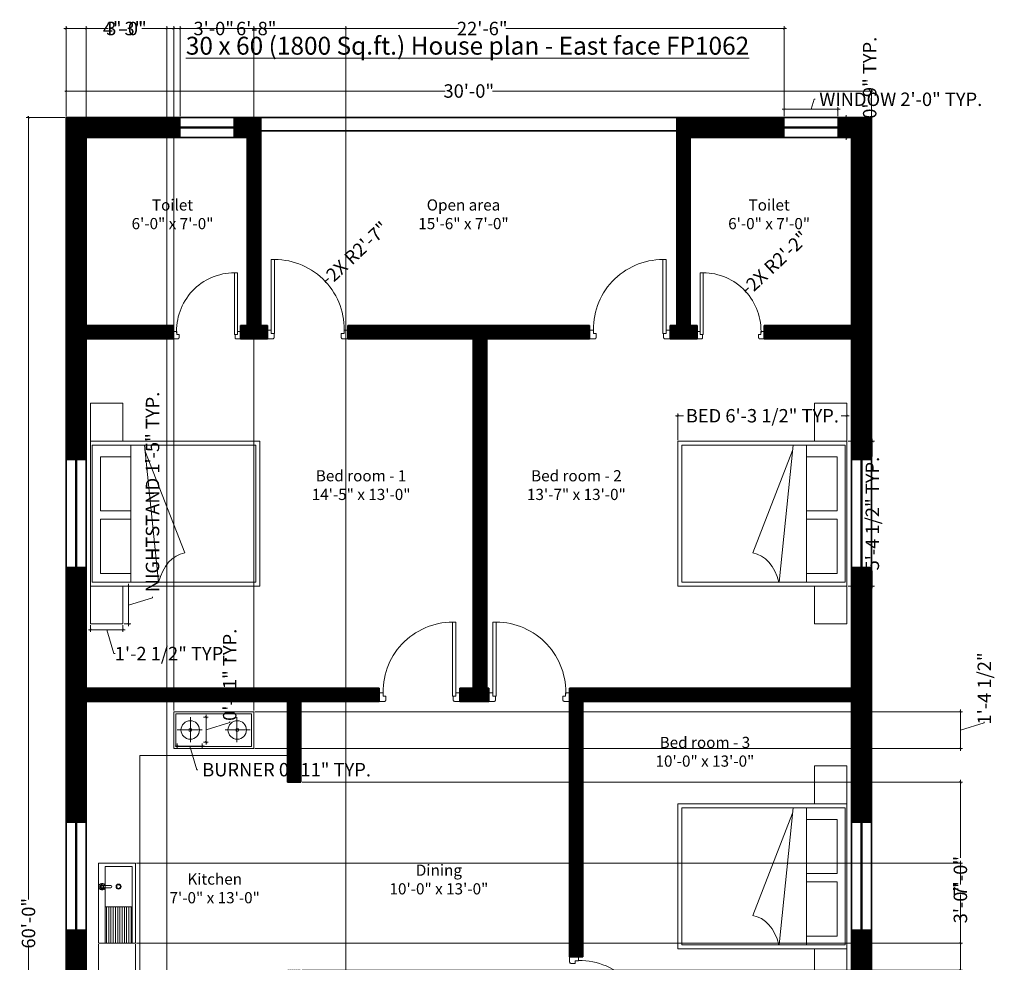
# Model space of a CAD drawing. Units: inches. Extents: x 111008 to 118198, y -138546 to -137723.
# Tile 4 of 4: x 117758 to 118198, y -138144 to -137723. Entities that reach past the tile are written whole.
import ezdxf

# ---------------------------------------------------------------- set-up
doc = ezdxf.new("R2010")
doc.units = ezdxf.units.IN
doc.header["$LTSCALE"] = 20
doc.header["$MEASUREMENT"] = 0
doc.header["$PDMODE"] = 3
for name, color, linetype, lineweight in [('A-ANNO-DIMS', 2, 'Continuous', 18), ('A-ANNO-TEXT', 7, 'Continuous', 18), ('A-AREA-IDEN', 7, 'Continuous', 18), ('A-DOOR', 181, 'Continuous', 18), ('A-EQPM', 7, 'Continuous', 18), ('A-FLOR-CASE', 181, 'Continuous', 18), ('A-FLOR-FIXT', 181, 'Continuous', 15), ('A-FLOR-FIXT-PATT', 181, 'Continuous', 9), ('ele', 6, 'Continuous', 20), ('furn', 181, 'Continuous', 15), ('FURNITURE', 8, 'Continuous', 15), ('FURNITURE - A', 6, 'Continuous', 0), ('walls', 7, 'Continuous', 35), ('WIN', 181, 'Continuous', 18)]:
    doc.layers.add(name, color=color, linetype=linetype, lineweight=lineweight)
doc.layers.add('A-WALL-PATT', color=251, linetype='Continuous', lineweight=9, true_color=0x636466)
doc.styles.add('vn1', font='arial.ttf', dxfattribs={"height": 6})
doc.dimstyles.new('vn1', dxfattribs={"dimtxt": 6, "dimasz": 1, "dimexe": 1, "dimexo": 0.5, "dimgap": 0.25, "dimtad": 0, "dimdec": 1, "dimzin": 3, "dimdsep": 46, "dimlunit": 4, "dimtxsty": 'vn1', "dimblk": 'ARCHTICK', "dimcen": 0, "dimdle": 1, "dimclrd": 8, "dimclre": 8, "dimclrt": 7, "dimadec": 0, "dimazin": 0, "dimtfac": 0.75, "dimtdec": 1, "dimtofl": 0, "dimtmove": 1, "dimatfit": 3, "dimfxl": 1, "dimtolj": 1, "dimtzin": 0, "dimlwd": -1, "dimlwe": -1, "dimarcsym": 0})

# ---------------------------------------------------------------- blocks, each defined once
blk = doc.blocks.new('_ArchTick')
at = {"color": 0, "linetype": 'ByBlock', "const_width": 0.15}
blk.add_lwpolyline([(-0.5, -0.5), (0.5, 0.5)], dxfattribs=at)
blk = doc.blocks.new('*D4')
at = {"layer": 'A-ANNO-DIMS', "color": 0, "transparency": 16777216}
for p, q in [((117778.41, -137766.56), (117761.13, -137766.56)), ((117762.13, -137766.06), (117762.13, -138115.99)), ((117762.13, -138487.06), (117762.13, -138137.13)), ((117778.41, -138486.56), (117761.13, -138486.56))]:
    blk.add_line(p, q, dxfattribs=at)
at = {"layer": 'Defpoints', "color": 0, "transparency": 16777216}
for p in [(117762.13, -137766.56), (117778.91, -137766.56), (117778.91, -138486.56)]:
    blk.add_point(p, dxfattribs=at)
at = {"layer": 'A-ANNO-DIMS', "color": 0, "transparency": 16777216}
for p, rotation in [((117762.13, -137766.56), 90), ((117762.13, -138486.56), 270)]:
    blk.add_blockref('_ArchTick', p, dxfattribs=dict(at, rotation=rotation))
at = {"layer": 'A-ANNO-DIMS', "color": 0, "transparency": 16777216, "insert": (117762.13, -138126.56), "char_height": 6, "attachment_point": 5, "rotation": 90, "style": 'vn1'}
blk.add_mtext('\\A1;60\'-0"', dxfattribs=at)
blk = doc.blocks.new('*D5')
at = {"layer": 'A-ANNO-DIMS', "color": 0, "transparency": 16777216}
for p, q in [((117778.41, -137754.78), (117948.35, -137754.78)), ((117778.91, -137766.06), (117778.91, -137753.78)), ((118139.41, -137754.78), (117969.46, -137754.78)), ((118138.91, -137766.06), (118138.91, -137753.78))]:
    blk.add_line(p, q, dxfattribs=at)
at = {"layer": 'Defpoints', "color": 0, "transparency": 16777216}
for p in [(118138.91, -137754.78), (117778.91, -137766.56), (118138.91, -137766.56)]:
    blk.add_point(p, dxfattribs=at)
at = {"layer": 'A-ANNO-DIMS', "color": 0, "transparency": 16777216, "rotation": 180}
blk.add_blockref('_ArchTick', (117778.91, -137754.78), dxfattribs=at)
at = {"layer": 'A-ANNO-DIMS', "color": 0, "transparency": 16777216}
blk.add_blockref('_ArchTick', (118138.91, -137754.78), dxfattribs=at)
at = {"layer": 'A-ANNO-DIMS', "color": 0, "transparency": 16777216, "insert": (117958.91, -137754.78), "char_height": 6, "attachment_point": 5, "style": 'vn1'}
blk.add_mtext('\\A1;30\'-0"', dxfattribs=at)
blk = doc.blocks.new('39 door')
at = {"layer": 'ele'}
blk.add_lwpolyline([(-17.62, 38.46), (-17.62, 2.69), (-16, 2.69), (-16, 38.46)], close=True, dxfattribs=at)
at = {"layer": 'furn'}
for points in [[(-16.87, 0), (-19.5, 0), (-19.5, 0), (-19.5, 4.31), (-17.62, 4.31), (-17.62, 2.69), (-16.27, 2.69), (-16.27, 0.6), (-16.42, 0.6), (-16.42, 0.45, -0.414214), (-16.72, 0.15), (-16.87, 0.15)], [(16.87, 0), (19.5, 0), (19.5, 0), (19.5, 4.31), (17.62, 4.31), (17.62, 2.69), (16.27, 2.69), (16.27, 0.6), (16.42, 0.6), (16.42, 0.45, 0.414214), (16.72, 0.15), (16.87, 0.15)]]:
    blk.add_lwpolyline(points, format="xyb", close=True, dxfattribs=at)
at = {"layer": 'WIN', "ltscale": 0.25}
blk.add_arc((-16.03, 4.75), 33.71, 356.5003, 89.9437, dxfattribs=at)
blk = doc.blocks.new('Bed 6')
at = {"layer": 'FURNITURE'}
for p, q in [((0, 35.96), (0, -35.96)), ((20.02, -33.97), (20.02, 34.04)), ((26.71, 34.01), (33.74, -34.02)), ((46.7, -19.51), (26.96, 31.37)), ((4.87, 1.37), (4.87, 28.24)), ((4.87, 28.24), (20.02, 28.24)), ((4.87, 1.37), (20.16, 1.37)), ((4.87, -2.82), (4.87, -29.7)), ((4.87, -2.82), (20.16, -2.82)), ((4.87, -29.7), (20.02, -29.7))]:
    blk.add_line(p, q, dxfattribs=at)
blk.add_ellipse((48.85, -42.03), major_axis=(-0.8, 22.65), ratio=0.705545, start_param=0.085096, end_param=1.184937, dxfattribs=at)
at = {"layer": 'FURNITURE - A'}
for p, q in [((0, 35.96), (84, 35.96)), ((84, 35.96), (84, -35.96)), ((0.81, -33.99), (0.81, 34.03)), ((0.81, 34.03), (81.97, 34.03)), ((81.97, 34.03), (81.97, -33.99)), ((81.97, -33.99), (0.81, -33.99)), ((84, -35.96), (0, -35.96))]:
    blk.add_line(p, q, dxfattribs=at)
blk = doc.blocks.new('WIN-48IN')
at = {"ltscale": 0.5}
for p, q in [((0, 48), (0, 0)), ((9, 48), (9, 0))]:
    blk.add_line(p, q, dxfattribs=at)
for p, q in [((0, 48), (9, 48)), ((0, 0), (9, 0))]:
    blk.add_line(p, q)
at = {"ltscale": 0.5, "const_width": 1}
blk.add_lwpolyline([(4.49, 48), (4.49, 0)], dxfattribs=at)
blk = doc.blocks.new('WIN-24IN')
at = {"ltscale": 0.5}
for p, q in [((0, 24), (0, 0)), ((9, 24), (9, 0))]:
    blk.add_line(p, q, dxfattribs=at)
for p, q in [((0, 24), (9, 24)), ((0, 0), (9, 0))]:
    blk.add_line(p, q)
at = {"ltscale": 0.5, "const_width": 1}
blk.add_lwpolyline([(4.49, 24), (4.49, 0)], dxfattribs=at)
blk = doc.blocks.new('BEDSIDE-TABLE')
blk.add_lwpolyline([(0, 16.95), (0, 0), (14.43, 0), (14.43, 16.95)], close=True)
blk = doc.blocks.new('COOKTOP-BURNER')
for p, q in [((5.91, 11.19), (5.91, 0)), ((0, 5.48), (11.19, 5.48))]:
    blk.add_line(p, q)
for radius in [4.13, 0.666]:
    blk.add_circle((5.79, 5.48), radius)
blk = doc.blocks.new('*D17')
at = {"layer": 'A-ANNO-DIMS', "color": 8, "transparency": 16777216}
for p, q in [((118111.91, -137762.96), (118113.25, -137758.48)), ((118113.25, -137758.48), (118113.75, -137758.48)), ((118098.91, -137762.96), (118124.91, -137762.96)), ((118099.91, -137766.06), (118099.91, -137761.96)), ((118123.91, -137766.06), (118123.91, -137761.96))]:
    blk.add_line(p, q, dxfattribs=at)
at = {"layer": 'Defpoints', "color": 0, "transparency": 16777216}
for p in [(118123.91, -137762.96), (118099.91, -137766.56), (118123.91, -137766.56)]:
    blk.add_point(p, dxfattribs=at)
at = {"layer": 'A-ANNO-DIMS', "color": 8, "transparency": 16777216, "rotation": 180}
blk.add_blockref('_ArchTick', (118099.91, -137762.96), dxfattribs=at)
at = {"layer": 'A-ANNO-DIMS', "color": 8, "transparency": 16777216}
blk.add_blockref('_ArchTick', (118123.91, -137762.96), dxfattribs=at)
at = {"layer": 'A-ANNO-DIMS', "color": 7, "transparency": 16777216, "insert": (118151.96, -137758.48), "char_height": 6, "attachment_point": 5, "style": 'vn1'}
blk.add_mtext('\\A1;WINDOW 2\'-0" TYP.', dxfattribs=at)
blk = doc.blocks.new('*D18')
at = {"layer": 'A-ANNO-DIMS', "color": 8, "transparency": 16777216}
for p, q in [((118124.41, -137766.56), (118128.51, -137766.56)), ((118127.51, -137765.56), (118127.51, -137776.56)), ((118127.51, -137771.06), (118138.07, -137767.89)), ((118138.07, -137767.89), (118138.07, -137767.39)), ((118124.41, -137775.56), (118128.51, -137775.56))]:
    blk.add_line(p, q, dxfattribs=at)
at = {"layer": 'Defpoints', "color": 0, "transparency": 16777216}
for p in [(118123.91, -137766.56), (118123.91, -137775.56), (118127.51, -137775.56)]:
    blk.add_point(p, dxfattribs=at)
at = {"layer": 'A-ANNO-DIMS', "color": 8, "transparency": 16777216}
for p, rotation in [((118127.51, -137766.56), 90), ((118127.51, -137775.56), 270)]:
    blk.add_blockref('_ArchTick', p, dxfattribs=dict(at, rotation=rotation))
at = {"layer": 'A-ANNO-DIMS', "color": 7, "transparency": 16777216, "insert": (118138.07, -137748.85), "char_height": 6, "attachment_point": 5, "rotation": 90, "style": 'vn1'}
blk.add_mtext('\\A1;0\'-9" TYP.', dxfattribs=at)
blk = doc.blocks.new('*D19')
at = {"layer": 'A-ANNO-DIMS', "color": 8, "transparency": 16777216}
for p, q in [((117806.88, -137993.88), (117806.88, -137974.93)), ((117804.84, -137975.93), (117807.88, -137975.93)), ((117806.88, -137984.4), (117817.56, -137981.2)), ((117817.56, -137981.2), (117817.56, -137980.7)), ((117804.84, -137992.88), (117807.88, -137992.88))]:
    blk.add_line(p, q, dxfattribs=at)
at = {"layer": 'Defpoints', "color": 0, "transparency": 16777216}
for p in [(117804.34, -137975.93), (117806.88, -137975.93), (117804.34, -137992.88)]:
    blk.add_point(p, dxfattribs=at)
at = {"layer": 'A-ANNO-DIMS', "color": 8, "transparency": 16777216}
for p, rotation in [((117806.88, -137975.93), 90), ((117806.88, -137992.88), 270)]:
    blk.add_blockref('_ArchTick', p, dxfattribs=dict(at, rotation=rotation))
at = {"layer": 'A-ANNO-DIMS', "color": 7, "transparency": 16777216, "insert": (117817.56, -137933.9), "char_height": 6, "attachment_point": 5, "rotation": 90, "style": 'vn1'}
blk.add_mtext('\\A1;NIGHTSTAND 1\'-5" TYP.', dxfattribs=at)
blk = doc.blocks.new('*D20')
at = {"layer": 'A-ANNO-DIMS', "color": 8, "transparency": 16777216}
for p, q in [((117788.91, -137995.42), (117805.34, -137995.42)), ((117789.91, -137993.38), (117789.91, -137996.42)), ((117797.12, -137995.42), (117800.33, -138006.1)), ((117804.34, -137993.38), (117804.34, -137996.42)), ((117800.33, -138006.1), (117800.83, -138006.1))]:
    blk.add_line(p, q, dxfattribs=at)
at = {"layer": 'Defpoints', "color": 0, "transparency": 16777216}
for p in [(117789.91, -137992.88), (117804.34, -137992.88), (117804.34, -137995.42)]:
    blk.add_point(p, dxfattribs=at)
at = {"layer": 'A-ANNO-DIMS', "color": 8, "transparency": 16777216, "rotation": 180}
blk.add_blockref('_ArchTick', (117789.91, -137995.42), dxfattribs=at)
at = {"layer": 'A-ANNO-DIMS', "color": 8, "transparency": 16777216}
blk.add_blockref('_ArchTick', (117804.34, -137995.42), dxfattribs=at)
at = {"layer": 'A-ANNO-DIMS', "color": 7, "transparency": 16777216, "insert": (117826.07, -138006.1), "char_height": 6, "attachment_point": 5, "style": 'vn1'}
blk.add_mtext('\\A1;1\'-2 1/2" TYP.', dxfattribs=at)
blk = doc.blocks.new('*D21')
at = {"layer": 'A-ANNO-DIMS', "color": 8, "transparency": 16777216}
for p, q in [((118051.31, -137899.85), (118054.93, -137899.85)), ((118052.31, -137910.69), (118052.31, -137898.85)), ((118128.91, -137899.85), (118125.28, -137899.85)), ((118127.91, -137910.69), (118127.91, -137898.85))]:
    blk.add_line(p, q, dxfattribs=at)
at = {"layer": 'Defpoints', "color": 0, "transparency": 16777216}
for p in [(118052.31, -137899.85), (118052.31, -137911.19), (118127.91, -137911.19)]:
    blk.add_point(p, dxfattribs=at)
at = {"layer": 'A-ANNO-DIMS', "color": 8, "transparency": 16777216, "rotation": 180}
blk.add_blockref('_ArchTick', (118052.31, -137899.85), dxfattribs=at)
at = {"layer": 'A-ANNO-DIMS', "color": 8, "transparency": 16777216}
blk.add_blockref('_ArchTick', (118127.91, -137899.85), dxfattribs=at)
at = {"layer": 'A-ANNO-DIMS', "color": 7, "transparency": 16777216, "insert": (118090.11, -137899.85), "char_height": 6, "attachment_point": 5, "style": 'vn1'}
blk.add_mtext('\\A1;BED 6\'-3 1/2" TYP.', dxfattribs=at)
blk = doc.blocks.new('*D22')
at = {"layer": 'A-ANNO-DIMS', "color": 8, "transparency": 16777216}
for p, q in [((118128.41, -137911.19), (118140.25, -137911.19)), ((118139.25, -137910.19), (118139.25, -137918.03)), ((118139.25, -137976.93), (118139.25, -137969.08)), ((118128.41, -137975.93), (118140.25, -137975.93))]:
    blk.add_line(p, q, dxfattribs=at)
at = {"layer": 'Defpoints', "color": 0, "transparency": 16777216}
for p in [(118127.91, -137911.19), (118139.25, -137911.19), (118127.91, -137975.93)]:
    blk.add_point(p, dxfattribs=at)
at = {"layer": 'A-ANNO-DIMS', "color": 8, "transparency": 16777216}
for p, rotation in [((118139.25, -137911.19), 90), ((118139.25, -137975.93), 270)]:
    blk.add_blockref('_ArchTick', p, dxfattribs=dict(at, rotation=rotation))
at = {"layer": 'A-ANNO-DIMS', "color": 7, "transparency": 16777216, "insert": (118139.25, -137943.56), "char_height": 6, "attachment_point": 5, "rotation": 90, "style": 'vn1'}
blk.add_mtext('\\A1;5\'-4 1/2" TYP.', dxfattribs=at)
blk = doc.blocks.new('*D23')
at = {"layer": 'A-ANNO-DIMS', "color": 8, "transparency": 16777216}
for p, q in [((117827.61, -138047.39), (117840.81, -138047.39)), ((117828.61, -138046.21), (117828.61, -138048.39)), ((117834.21, -138047.39), (117837.38, -138057.96)), ((117839.81, -138046.21), (117839.81, -138048.39)), ((117837.38, -138057.96), (117837.88, -138057.96))]:
    blk.add_line(p, q, dxfattribs=at)
at = {"layer": 'Defpoints', "color": 0, "transparency": 16777216}
for p in [(117828.61, -138045.71), (117839.81, -138045.71), (117839.81, -138047.39)]:
    blk.add_point(p, dxfattribs=at)
at = {"layer": 'A-ANNO-DIMS', "color": 8, "transparency": 16777216, "rotation": 180}
blk.add_blockref('_ArchTick', (117828.61, -138047.39), dxfattribs=at)
at = {"layer": 'A-ANNO-DIMS', "color": 8, "transparency": 16777216}
blk.add_blockref('_ArchTick', (117839.81, -138047.39), dxfattribs=at)
at = {"layer": 'A-ANNO-DIMS', "color": 7, "transparency": 16777216, "insert": (117877.47, -138057.96), "char_height": 6, "attachment_point": 5, "style": 'vn1'}
blk.add_mtext('\\A1;BURNER 0\'-11" TYP.', dxfattribs=at)
blk = doc.blocks.new('*D24')
at = {"layer": 'A-ANNO-DIMS', "color": 8, "transparency": 16777216}
for p, q in [((117840.31, -138034.52), (117842.49, -138034.52)), ((117841.49, -138046.71), (117841.49, -138033.52)), ((117841.49, -138040.12), (117852.05, -138036.95)), ((117852.05, -138036.95), (117852.05, -138036.45)), ((117840.31, -138045.71), (117842.49, -138045.71))]:
    blk.add_line(p, q, dxfattribs=at)
at = {"layer": 'Defpoints', "color": 0, "transparency": 16777216}
for p in [(117839.81, -138034.52), (117841.49, -138034.52), (117839.81, -138045.71)]:
    blk.add_point(p, dxfattribs=at)
at = {"layer": 'A-ANNO-DIMS', "color": 8, "transparency": 16777216}
for p, rotation in [((117841.49, -138034.52), 90), ((117841.49, -138045.71), 270)]:
    blk.add_blockref('_ArchTick', p, dxfattribs=dict(at, rotation=rotation))
at = {"layer": 'A-ANNO-DIMS', "color": 7, "transparency": 16777216, "insert": (117852.05, -138015.58), "char_height": 6, "attachment_point": 5, "rotation": 90, "style": 'vn1'}
blk.add_mtext('\\A1;0\'-11" TYP.', dxfattribs=at)
blk = doc.blocks.new('*D26')
at = {"layer": 'A-ANNO-DIMS', "color": 8, "transparency": 16777216}
for p, q in [((118178.61, -138062.56), (118178.61, -138097.36)), ((117884.41, -138063.56), (118179.61, -138063.56)), ((118178.61, -138148.56), (118178.61, -138113.76)), ((117884.41, -138147.56), (118179.61, -138147.56))]:
    blk.add_line(p, q, dxfattribs=at)
at = {"layer": 'Defpoints', "color": 0, "transparency": 16777216}
for p in [(117883.91, -138063.56), (117883.91, -138147.56), (118178.61, -138147.56)]:
    blk.add_point(p, dxfattribs=at)
at = {"layer": 'A-ANNO-DIMS', "color": 8, "transparency": 16777216}
for p, rotation in [((118178.61, -138063.56), 90), ((118178.61, -138147.56), 270)]:
    blk.add_blockref('_ArchTick', p, dxfattribs=dict(at, rotation=rotation))
at = {"layer": 'A-ANNO-DIMS', "color": 7, "transparency": 16777216, "insert": (118178.61, -138105.56), "char_height": 6, "attachment_point": 5, "rotation": 90, "style": 'vn1'}
blk.add_mtext('\\A1;7\'-0"', dxfattribs=at)
blk = doc.blocks.new('*D27')
at = {"layer": 'A-ANNO-DIMS', "color": 8, "transparency": 16777216}
for p, q in [((117793.41, -138135.94), (117793.41, -138527.26)), ((117809.91, -138135.94), (117809.91, -138527.26)), ((117792.41, -138526.26), (117810.91, -138526.26)), ((117801.66, -138526.26), (117804.86, -138536.94)), ((117804.86, -138536.94), (117805.36, -138536.94))]:
    blk.add_line(p, q, dxfattribs=at)
at = {"layer": 'Defpoints', "color": 0, "transparency": 16777216}
for p in [(117793.41, -138135.44), (117809.91, -138135.44), (117809.91, -138526.26)]:
    blk.add_point(p, dxfattribs=at)
at = {"layer": 'A-ANNO-DIMS', "color": 8, "transparency": 16777216, "rotation": 180}
blk.add_blockref('_ArchTick', (117793.41, -138526.26), dxfattribs=at)
at = {"layer": 'A-ANNO-DIMS', "color": 8, "transparency": 16777216}
blk.add_blockref('_ArchTick', (117809.91, -138526.26), dxfattribs=at)
at = {"layer": 'A-ANNO-DIMS', "color": 7, "transparency": 16777216, "insert": (117820.29, -138536.94), "char_height": 6, "attachment_point": 5, "style": 'vn1'}
blk.add_mtext('\\A1;1\'-4 1/2"', dxfattribs=at)
blk = doc.blocks.new('*D28')
at = {"layer": 'A-ANNO-DIMS', "color": 8, "transparency": 16777216}
for p, q in [((117810.41, -138099.68), (118179.61, -138099.68)), ((118178.61, -138098.68), (118178.61, -138109.33)), ((118178.61, -138136.44), (118178.61, -138125.78)), ((117810.41, -138135.44), (118179.61, -138135.44))]:
    blk.add_line(p, q, dxfattribs=at)
at = {"layer": 'Defpoints', "color": 0, "transparency": 16777216}
for p in [(117809.91, -138099.68), (118178.61, -138099.68), (117809.91, -138135.44)]:
    blk.add_point(p, dxfattribs=at)
at = {"layer": 'A-ANNO-DIMS', "color": 8, "transparency": 16777216}
for p, rotation in [((118178.61, -138099.68), 90), ((118178.61, -138135.44), 270)]:
    blk.add_blockref('_ArchTick', p, dxfattribs=dict(at, rotation=rotation))
at = {"layer": 'A-ANNO-DIMS', "color": 7, "transparency": 16777216, "insert": (118178.61, -138117.56), "char_height": 6, "attachment_point": 5, "rotation": 90, "style": 'vn1'}
blk.add_mtext('\\A1;3\'-0"', dxfattribs=at)
blk = doc.blocks.new('*D29')
at = {"layer": 'A-ANNO-DIMS', "color": 8, "transparency": 16777216}
for p, q in [((117826.03, -137726.86), (117836.68, -137726.86)), ((117827.03, -138031.56), (117827.03, -137725.86)), ((117863.79, -137726.86), (117853.13, -137726.86)), ((117862.79, -138031.56), (117862.79, -137725.86))]:
    blk.add_line(p, q, dxfattribs=at)
at = {"layer": 'Defpoints', "color": 0, "transparency": 16777216}
for p in [(117862.79, -137726.86), (117827.03, -138032.06), (117862.79, -138032.06)]:
    blk.add_point(p, dxfattribs=at)
at = {"layer": 'A-ANNO-DIMS', "color": 8, "transparency": 16777216, "rotation": 180}
blk.add_blockref('_ArchTick', (117827.03, -137726.86), dxfattribs=at)
at = {"layer": 'A-ANNO-DIMS', "color": 8, "transparency": 16777216}
blk.add_blockref('_ArchTick', (117862.79, -137726.86), dxfattribs=at)
at = {"layer": 'A-ANNO-DIMS', "color": 7, "transparency": 16777216, "insert": (117844.91, -137726.86), "char_height": 6, "attachment_point": 5, "style": 'vn1'}
blk.add_mtext('\\A1;3\'-0"', dxfattribs=at)
blk = doc.blocks.new('*D30')
at = {"layer": 'A-ANNO-DIMS', "color": 8, "transparency": 16777216}
for p, q in [((117863.29, -138032.06), (118179.61, -138032.06)), ((118178.61, -138049.56), (118178.61, -138031.06)), ((118189.29, -138037.1), (118189.29, -138036.6)), ((118178.61, -138040.31), (118189.29, -138037.1)), ((117863.29, -138048.56), (118179.61, -138048.56))]:
    blk.add_line(p, q, dxfattribs=at)
at = {"layer": 'Defpoints', "color": 0, "transparency": 16777216}
for p in [(117862.79, -138032.06), (118178.61, -138032.06), (117862.79, -138048.56)]:
    blk.add_point(p, dxfattribs=at)
at = {"layer": 'A-ANNO-DIMS', "color": 8, "transparency": 16777216}
for p, rotation in [((118178.61, -138032.06), 90), ((118178.61, -138048.56), 270)]:
    blk.add_blockref('_ArchTick', p, dxfattribs=dict(at, rotation=rotation))
at = {"layer": 'A-ANNO-DIMS', "color": 7, "transparency": 16777216, "insert": (118189.29, -138021.67), "char_height": 6, "attachment_point": 5, "rotation": 90, "style": 'vn1'}
blk.add_mtext('\\A1;1\'-4 1/2"', dxfattribs=at)
blk = doc.blocks.new('*D33')
at = {"layer": 'A-ANNO-DIMS', "color": 8, "transparency": 16777216}
for p, q in [((117786.91, -137726.86), (117797.68, -137726.86)), ((117787.91, -138228.06), (117787.91, -137725.86)), ((117824.91, -137726.86), (117814.13, -137726.86)), ((117823.91, -138228.06), (117823.91, -137725.86))]:
    blk.add_line(p, q, dxfattribs=at)
at = {"layer": 'Defpoints', "color": 0, "transparency": 16777216}
for p in [(117823.91, -137726.86), (117787.91, -138228.56), (117823.91, -138228.56)]:
    blk.add_point(p, dxfattribs=at)
at = {"layer": 'A-ANNO-DIMS', "color": 8, "transparency": 16777216, "rotation": 180}
blk.add_blockref('_ArchTick', (117787.91, -137726.86), dxfattribs=at)
at = {"layer": 'A-ANNO-DIMS', "color": 8, "transparency": 16777216}
blk.add_blockref('_ArchTick', (117823.91, -137726.86), dxfattribs=at)
at = {"layer": 'A-ANNO-DIMS', "color": 7, "transparency": 16777216, "insert": (117805.91, -137726.86), "char_height": 6, "attachment_point": 5, "style": 'vn1'}
blk.add_mtext('\\A1;3\'-0"', dxfattribs=at)
blk = doc.blocks.new('*D34')
at = {"layer": 'A-ANNO-DIMS', "color": 8, "transparency": 16777216}
for p, q in [((117822.91, -137726.86), (117855.67, -137726.86)), ((117823.91, -138226.06), (117823.91, -137725.86)), ((117904.91, -137726.86), (117872.15, -137726.86)), ((117903.91, -138226.06), (117903.91, -137725.86))]:
    blk.add_line(p, q, dxfattribs=at)
at = {"layer": 'Defpoints', "color": 0, "transparency": 16777216}
for p in [(117903.91, -137726.86), (117823.91, -138226.56), (117903.91, -138226.56)]:
    blk.add_point(p, dxfattribs=at)
at = {"layer": 'A-ANNO-DIMS', "color": 8, "transparency": 16777216, "rotation": 180}
blk.add_blockref('_ArchTick', (117823.91, -137726.86), dxfattribs=at)
at = {"layer": 'A-ANNO-DIMS', "color": 8, "transparency": 16777216}
blk.add_blockref('_ArchTick', (117903.91, -137726.86), dxfattribs=at)
at = {"layer": 'A-ANNO-DIMS', "color": 7, "transparency": 16777216, "insert": (117863.91, -137726.86), "char_height": 6, "attachment_point": 5, "style": 'vn1'}
blk.add_mtext('\\A1;6\'-8"', dxfattribs=at)
blk = doc.blocks.new('*D36')
at = {"layer": 'A-ANNO-DIMS', "color": 8, "transparency": 16777216}
for p, q in [((117828.91, -137726.86), (117954.3, -137726.86)), ((117829.91, -137766.06), (117829.91, -137725.86)), ((118100.91, -137726.86), (117975.51, -137726.86)), ((118099.91, -137766.06), (118099.91, -137725.86))]:
    blk.add_line(p, q, dxfattribs=at)
at = {"layer": 'Defpoints', "color": 0, "transparency": 16777216}
for p in [(118099.91, -137726.86), (117829.91, -137766.56), (118099.91, -137766.56)]:
    blk.add_point(p, dxfattribs=at)
at = {"layer": 'A-ANNO-DIMS', "color": 8, "transparency": 16777216, "rotation": 180}
blk.add_blockref('_ArchTick', (117829.91, -137726.86), dxfattribs=at)
at = {"layer": 'A-ANNO-DIMS', "color": 8, "transparency": 16777216}
blk.add_blockref('_ArchTick', (118099.91, -137726.86), dxfattribs=at)
at = {"layer": 'A-ANNO-DIMS', "color": 7, "transparency": 16777216, "insert": (117964.91, -137726.86), "char_height": 6, "attachment_point": 5, "style": 'vn1'}
blk.add_mtext('\\A1;22\'-6"', dxfattribs=at)
blk = doc.blocks.new('*D37')
at = {"layer": 'A-ANNO-DIMS', "color": 8, "transparency": 16777216}
for p, q in [((117777.91, -137726.86), (117796.06, -137726.86)), ((117778.91, -137766.06), (117778.91, -137725.86)), ((117830.91, -137726.86), (117812.75, -137726.86)), ((117829.91, -137766.06), (117829.91, -137725.86))]:
    blk.add_line(p, q, dxfattribs=at)
at = {"layer": 'Defpoints', "color": 0, "transparency": 16777216}
for p in [(117829.91, -137726.86), (117778.91, -137766.56), (117829.91, -137766.56)]:
    blk.add_point(p, dxfattribs=at)
at = {"layer": 'A-ANNO-DIMS', "color": 8, "transparency": 16777216, "rotation": 180}
blk.add_blockref('_ArchTick', (117778.91, -137726.86), dxfattribs=at)
at = {"layer": 'A-ANNO-DIMS', "color": 8, "transparency": 16777216}
blk.add_blockref('_ArchTick', (117829.91, -137726.86), dxfattribs=at)
at = {"layer": 'A-ANNO-DIMS', "color": 7, "transparency": 16777216, "insert": (117804.41, -137726.86), "char_height": 6, "attachment_point": 5, "style": 'vn1'}
blk.add_mtext('\\A1;4\'-3"', dxfattribs=at)
blk = doc.blocks.new('*D38')
at = {"layer": 'A-ANNO-DIMS', "color": 8, "transparency": 16777216}
blk.add_line((117896.24, -137838.49), (117894.78, -137839.86), dxfattribs=at)
at = {"layer": 'Defpoints', "color": 0, "transparency": 16777216}
for p in [(117894.78, -137839.86), (117872.11, -137861.17)]:
    blk.add_point(p, dxfattribs=at)
at = {"layer": 'A-ANNO-DIMS', "color": 8, "transparency": 16777216, "rotation": 223.2214413739515}
blk.add_blockref('_ArchTick', (117894.78, -137839.86), dxfattribs=at)
at = {"layer": 'A-ANNO-DIMS', "color": 7, "transparency": 16777216, "insert": (117909.06, -137826.44), "char_height": 6, "attachment_point": 5, "rotation": 43.2214, "style": 'vn1'}
blk.add_mtext('\\A1;2X R2\'-7"', dxfattribs=at)
blk = doc.blocks.new('*D39')
at = {"layer": 'A-ANNO-DIMS', "color": 8, "transparency": 16777216}
blk.add_line((118083.93, -137842.77), (118082.47, -137844.14), dxfattribs=at)
at = {"layer": 'Defpoints', "color": 0, "transparency": 16777216}
for p in [(118082.47, -137844.14), (118063.57, -137861.9)]:
    blk.add_point(p, dxfattribs=at)
at = {"layer": 'A-ANNO-DIMS', "color": 8, "transparency": 16777216, "rotation": 223.2226867957486}
blk.add_blockref('_ArchTick', (118082.47, -137844.14), dxfattribs=at)
at = {"layer": 'A-ANNO-DIMS', "color": 7, "transparency": 16777216, "insert": (118096.75, -137830.73), "char_height": 6, "attachment_point": 5, "rotation": 43.2227, "style": 'vn1'}
blk.add_mtext('\\A1;2X R2\'-2"', dxfattribs=at)

msp = doc.modelspace()

# ---------------------------------------------------------------- hatches: boundary and pattern name
at = {"layer": 'A-FLOR-FIXT-PATT'}
h = msp.add_hatch(dxfattribs=at)
h.set_pattern_fill('ANSI31', color=256, scale=8, angle=45, style=0)
h.paths.add_polyline_path([(117796.41, -138135.44), (117808.41, -138135.44), (117808.41, -138119.18), (117796.41, -138119.18)])
at = {"layer": 'A-WALL-PATT'}
h = msp.add_hatch(dxfattribs=at)
h.set_pattern_fill('ANSI31', color=256)
h.paths.add_polyline_path([(117829.91, -137766.56), (117778.91, -137766.56), (117778.91, -137919.56), (117787.91, -137919.56), (117787.91, -137865.56), (117826.91, -137865.56), (117826.91, -137859.56), (117787.91, -137859.56), (117787.91, -137775.56), (117829.91, -137775.56)])
h.paths.add_polyline_path([(117865.91, -137766.56), (117853.91, -137766.56), (117853.91, -137775.56), (117859.91, -137775.56), (117859.91, -137859.56), (117856.91, -137859.56), (117856.91, -137865.56), (117868.91, -137865.56), (117868.91, -137861.58), (117868.91, -137859.56), (117865.91, -137859.56)])
h.paths.add_polyline_path([(118099.91, -137766.56), (118051.91, -137766.56), (118051.91, -137859.56), (118048.91, -137859.56), (118048.91, -137865.56), (118060.91, -137865.56), (118060.91, -137862.24), (118060.91, -137859.56), (118057.91, -137859.56), (118057.91, -137775.56), (118099.91, -137775.56)])
h.paths.add_polyline_path([(118138.91, -137766.56), (118123.91, -137766.56), (118123.91, -137775.56), (118129.91, -137775.56), (118129.91, -137859.56), (118090.91, -137859.56), (118090.91, -137865.56), (118129.91, -137865.56), (118129.91, -137919.56), (118138.91, -137919.56)])
h.paths.add_polyline_path([(118138.91, -137967.56), (118129.91, -137967.56), (118129.91, -138021.56), (118003.91, -138021.56), (118003.91, -138141.56), (118007.88, -138141.56), (118009.91, -138141.56), (118009.91, -138027.56), (118129.91, -138027.56), (118129.91, -138081.56), (118138.91, -138081.56)])
h.paths.add_polyline_path([(118012.91, -137861.58), (118012.91, -137859.56), (117904.91, -137859.56), (117904.91, -137865.56), (117960.91, -137865.56), (117960.91, -138021.56), (117954.91, -138021.56), (117954.91, -138027.56), (117967.91, -138027.56), (117967.91, -138023.58), (117967.91, -138021.56), (117966.91, -138021.56), (117966.91, -137865.56), (118012.91, -137865.56)])
h.paths.add_polyline_path([(117787.91, -138027.56), (117877.91, -138027.56), (117877.91, -138063.56), (117883.91, -138063.56), (117883.91, -138027.56), (117918.91, -138027.56), (117918.91, -138023.58), (117918.91, -138021.56), (117787.91, -138021.56), (117787.91, -137967.56), (117778.91, -137967.56), (117778.91, -138081.56), (117787.91, -138081.56)])
h.paths.add_polyline_path([(117787.91, -138129.56), (117778.91, -138129.56), (117778.91, -138204.56), (117787.91, -138204.56), (117787.91, -138189.56), (117899.91, -138189.56), (117899.91, -138185.58), (117899.91, -138183.56), (117883.91, -138183.56), (117883.91, -138147.56), (117877.91, -138147.56), (117877.91, -138183.56), (117787.91, -138183.56)])
h.paths.add_polyline_path([(118138.91, -138129.56), (118129.91, -138129.56), (118129.91, -138183.56), (118009.91, -138183.56), (118009.91, -138177.56), (118003.91, -138177.56), (118003.91, -138189.56), (118039.91, -138189.56), (118039.91, -138195.56), (118045.91, -138195.56), (118045.91, -138189.56), (118129.91, -138189.56), (118129.91, -138201.56), (118138.91, -138201.56)])
h.paths.add_polyline_path([(118138.91, -138225.56), (118129.91, -138225.56), (118129.91, -138237.56), (118045.91, -138237.56), (118045.91, -138225.56), (118043.2, -138225.56), (118043.2, -138225.56), (118039.91, -138225.56), (118039.91, -138243.56), (118129.91, -138243.56), (118129.91, -138301.06), (118138.91, -138301.06)])
h.paths.add_polyline_path([(117944.91, -138183.56), (117935.91, -138183.56), (117935.91, -138293.56), (117944.91, -138293.56)])
h.paths.add_polyline_path([(117899.91, -138267.56), (117787.91, -138267.56), (117787.91, -138252.56), (117778.91, -138252.56), (117778.91, -138486.56), (117787.91, -138486.56), (117787.91, -138276.56), (117899.91, -138276.56), (117899.91, -138272.58)])
h.paths.add_polyline_path([(117944.91, -138341.56), (117935.91, -138341.56), (117935.91, -138364.56), (117939.88, -138364.56), (117944.91, -138364.56)])
h.paths.add_polyline_path([(118011.91, -138406.56), (117941.91, -138406.56), (117941.91, -138400.56), (117935.91, -138400.56), (117935.91, -138415.56), (118011.91, -138415.56)], flags=17)
h.paths.add_polyline_path([(118138.91, -138349.06), (118129.91, -138349.06), (118129.91, -138406.56), (118059.91, -138406.56), (118059.91, -138415.56), (118129.91, -138415.56), (118129.91, -138477.56), (117935.91, -138477.56), (117935.91, -138486.56), (118138.91, -138486.56)])

# ---------------------------------------------------------------- linework, layer by layer
at = {"layer": 'A-EQPM'}
for points in [[(117862.79, -138048.56), (117862.79, -138032.06), (117827.03, -138032.06), (117827.03, -138048.56)], [(117861.79, -138047.56), (117861.79, -138033.06), (117828.03, -138033.06), (117828.03, -138047.56)]]:
    msp.add_lwpolyline(points, close=True, dxfattribs=at)
at = {"layer": 'A-FLOR-CASE'}
for p, q in [((117811.91, -138051.56), (117811.91, -138183.56)), ((117877.91, -138051.56), (117811.91, -138051.56))]:
    msp.add_line(p, q, dxfattribs=at)
at = {"layer": 'A-FLOR-FIXT'}
for p, q in [((117798.89, -138109.77), (117795.86, -138109.77)), ((117795.86, -138110.73), (117798.89, -138110.73))]:
    msp.add_line(p, q, dxfattribs=at)
at = {"layer": 'A-FLOR-FIXT', "ltscale": 0.1}
for p, q in [((117796.41, -138135.44), (117796.41, -138119.18)), ((117808.41, -138135.44), (117808.41, -138119.18))]:
    msp.add_line(p, q, dxfattribs=at)
at = {"layer": 'A-FLOR-FIXT'}
msp.add_lwpolyline([(117809.91, -138099.68), (117793.41, -138099.68), (117793.41, -138135.44), (117809.91, -138135.44)], close=True, dxfattribs=at)
at = {"layer": 'A-FLOR-FIXT', "ltscale": 0.1}
msp.add_lwpolyline([(117808.41, -138101.18), (117796.41, -138101.18), (117796.41, -138119.18), (117808.41, -138119.18)], close=True, dxfattribs=at)
at = {"layer": 'A-FLOR-FIXT'}
for centre, radius in [((117795.03, -138110.25), 0.718), ((117795.03, -138110.25), 0.479), ((117802.41, -138110.18), 1.12), ((117802.41, -138110.18), 0.844)]:
    msp.add_circle(centre, radius, dxfattribs=at)
for centre, radius, start, end in [((117795.03, -138110.25), 1.44, 19.6514, 340.3603), ((117795.03, -138110.25), 0.958, 30.3431, 329.7554), ((117798.89, -138110.25), 0.479, 270, 90)]:
    msp.add_arc(centre, radius, start, end, dxfattribs=at)
at = {"layer": 'walls'}
for p, q in [((117865.91, -137766.56), (117865.91, -137859.56)), ((117865.91, -137766.56), (118051.91, -137766.56)), ((118051.91, -137859.56), (118051.91, -137766.56)), ((117865.91, -137772.56), (118051.91, -137772.56)), ((117787.91, -137775.56), (117787.91, -137859.56)), ((117859.91, -137775.56), (117787.91, -137775.56)), ((117859.91, -137775.56), (117859.91, -137859.56)), ((118129.91, -137775.56), (118057.91, -137775.56)), ((118057.91, -137859.56), (118057.91, -137775.56)), ((118129.91, -137859.56), (118129.91, -137775.56)), ((117826.91, -137859.56), (117787.91, -137859.56)), ((117826.91, -137859.56), (117826.91, -137865.56)), ((117856.91, -137859.56), (117856.91, -137865.56)), ((117859.91, -137859.56), (117856.91, -137859.56)), ((117868.91, -137859.56), (117865.91, -137859.56)), ((117868.91, -137859.56), (117868.91, -137865.56)), ((117904.91, -137859.56), (117904.91, -137865.56)), ((118012.91, -137859.56), (117904.91, -137859.56)), ((118012.91, -137865.56), (118012.91, -137859.56)), ((118048.91, -137865.56), (118048.91, -137859.56)), ((118051.91, -137859.56), (118048.91, -137859.56)), ((118060.91, -137859.56), (118057.91, -137859.56)), ((118060.91, -137865.56), (118060.91, -137859.56)), ((118129.91, -137859.56), (118090.91, -137859.56)), ((118090.91, -137865.56), (118090.91, -137859.56)), ((117826.91, -137865.56), (117787.91, -137865.56)), ((117787.91, -137865.56), (117787.91, -138021.56)), ((117868.91, -137865.56), (117856.91, -137865.56)), ((117960.91, -137865.56), (117904.91, -137865.56)), ((117960.91, -137865.56), (117960.91, -138021.56)), ((117966.91, -137865.56), (117966.91, -138021.56)), ((118012.91, -137865.56), (117966.91, -137865.56)), ((118060.91, -137865.56), (118048.91, -137865.56)), ((118129.91, -137865.56), (118090.91, -137865.56)), ((118129.91, -138021.56), (118129.91, -137865.56)), ((117918.91, -138021.56), (117787.91, -138021.56)), ((117918.91, -138021.56), (117918.91, -138027.56)), ((117954.91, -138021.56), (117954.91, -138027.56)), ((117960.91, -138021.56), (117954.91, -138021.56)), ((117967.91, -138021.56), (117966.91, -138021.56)), ((117967.91, -138027.56), (117967.91, -138021.56)), ((118129.91, -138021.56), (118003.91, -138021.56)), ((118003.91, -138141.56), (118003.91, -138021.56)), ((117877.91, -138027.56), (117787.91, -138027.56)), ((117787.91, -138027.56), (117787.91, -138183.56)), ((117877.91, -138027.56), (117877.91, -138063.56)), ((117883.91, -138027.56), (117883.91, -138063.56)), ((117918.91, -138027.56), (117883.91, -138027.56)), ((117967.91, -138027.56), (117954.91, -138027.56)), ((118129.91, -138027.56), (118009.91, -138027.56)), ((118009.91, -138141.56), (118009.91, -138027.56)), ((118129.91, -138183.56), (118129.91, -138027.56)), ((117883.91, -138063.56), (117877.91, -138063.56)), ((118009.91, -138141.56), (118003.91, -138141.56))]:
    msp.add_line(p, q, dxfattribs=at)
for points in [[(117865.91, -137766.56), (117778.91, -137766.56), (117778.91, -138486.56), (117787.91, -138486.56)], [(117935.91, -138486.56), (118138.91, -138486.56), (118138.91, -137766.56), (118051.91, -137766.56)]]:
    msp.add_lwpolyline(points, dxfattribs=at)

# ---------------------------------------------------------------- block references
at = {"layer": 'A-DOOR', "ltscale": 0.15}
for p, xscale, yscale, zscale in [((117886.91, -137865.56), 0.9230769230771328, 0.9230769230771328, 0.9230769230771328), ((118030.91, -137865.56), -0.9230769230771328, 0.9230769230771328, 0.9230769230771328), ((117841.91, -137865.56), -0.7692306364006699, 0.7692306364006699, 0.7692306364006699), ((118075.91, -137865.56), 0.7692306364006699, 0.7692306364006699, 0.7692306364006699), ((117936.91, -138027.56), -0.9230769230771328, 0.9230769230771328, 0.9230769230771328), ((117985.91, -138027.56), 0.9230769230771328, 0.9230769230771328, 0.9230769230771328)]:
    msp.add_blockref('39 door', p, dxfattribs=dict(at, xscale=xscale, yscale=yscale, zscale=zscale))
at = {"layer": 'A-DOOR', "ltscale": 0.15, "xscale": -0.9230769230771328, "yscale": 0.9230769230771328, "zscale": 0.9230769230771328, "rotation": 270}
msp.add_blockref('39 door', (118003.91, -138159.56), dxfattribs=at)
at = {"layer": 'A-EQPM'}
msp.add_blockref('COOKTOP-BURNER', (117828.61, -138045.71), dxfattribs=at)
at = {"layer": 'A-EQPM', "extrusion": (0, 0, -1), "zscale": -1}
msp.add_blockref('COOKTOP-BURNER', (-117861.2, -138045.71), dxfattribs=at)
at = {"layer": 'FURNITURE', "extrusion": (0, 0, -1), "zscale": -1, "rotation": 180}
msp.add_blockref('BEDSIDE-TABLE', (-117789.91, -137894.24), dxfattribs=at)
at = {"layer": 'FURNITURE', "rotation": 180}
for p in [(118127.91, -137894.24), (118127.91, -138056.24)]:
    msp.add_blockref('BEDSIDE-TABLE', p, dxfattribs=at)
at = {"layer": 'FURNITURE', "yscale": 0.900000000000091, "zscale": 0.900000000000091}
for p, xscale in [((117789.91, -137943.56), 0.900000000000091), ((118127.91, -137943.56), -0.900000000000091), ((118127.91, -138105.56), -0.900000000000091)]:
    msp.add_blockref('Bed 6', p, dxfattribs=dict(at, xscale=xscale))
at = {"layer": 'FURNITURE'}
msp.add_blockref('BEDSIDE-TABLE', (117789.91, -137992.88), dxfattribs=at)
at = {"layer": 'FURNITURE', "extrusion": (0, 0, -1), "zscale": -1}
for p in [(-118127.91, -137992.88), (-118127.91, -138154.88)]:
    msp.add_blockref('BEDSIDE-TABLE', p, dxfattribs=at)
at = {"layer": 'WIN'}
for p, rotation in [((117829.91, -137766.56), 270.0000000003883), ((118099.91, -137766.56), 270.000000000434)]:
    msp.add_blockref('WIN-24IN', p, dxfattribs=dict(at, rotation=rotation))
for p in [(117778.91, -137967.56), (118129.91, -137967.56), (117778.91, -138129.56), (118129.91, -138129.56)]:
    msp.add_blockref('WIN-48IN', p, dxfattribs=at)

# ---------------------------------------------------------------- texts
at = {"layer": 'A-ANNO-TEXT', "insert": (117824.84, -137730.54), "char_height": 8, "attachment_point": 1, "style": 'vn1'}
msp.add_mtext_dynamic_manual_height_columns('\\pxqc;{\\fArial|b1|i0|c0|p34;\\L30 x 60 (1800 Sq.ft.) House plan - East face FP1062}', width=266.9998, gutter_width=30, heights=[0], dxfattribs=at)
at = {"layer": 'A-AREA-IDEN', "char_height": 5, "attachment_point": 1, "style": 'vn1'}
for s, insert in [('\\pxqc;Toilet\\P6\'-0" x 7\'-0"', (117799.18, -137803.18)), ('\\pxqc;Open area\\P15\'-6" x 7\'-0"', (117929.22, -137803.18)), ('\\pxqc;Toilet\\P6\'-0" x 7\'-0"', (118065.81, -137803.18)), ('\\pxqc;Bed room - 1\\P14\'-5" x 13\'-0"', (117883.47, -137924.16)), ('\\pxqc;Bed room - 2\\P13\'-7" x 13\'-0"', (117979.68, -137924.16)), ('\\pxqc;Bed room - 3\\P10\'-0" x 13\'-0"', (118037.12, -138043.29)), ('\\pxqc;Dining\\P10\'-0" x 13\'-0"', (117918.24, -138100.36)), ('\\pxqc;Kitchen\\P7\'-0" x 13\'-0"', (117818.03, -138104.33))]:
    msp.add_mtext_dynamic_manual_height_columns(s, width=54.6246, gutter_width=30, heights=[0], dxfattribs=dict(at, insert=insert))

# ---------------------------------------------------------------- dimensions: what is measured, and where the dimension line sits
at = {"layer": 'A-ANNO-DIMS'}
for base, p1, p2, override, picture, middle in [((117829.91, -137726.86), (117778.91, -137766.56), (117829.91, -137766.56), {"dimdec": 1, "dimlfac": 1, "dimrnd": 0, "dimzin": 1, "dimdsep": 46, "dimlunit": 4, "dimfrac": 2}, '*D37', (117804.41, -137726.86)), ((117823.91, -137726.86), (117787.91, -138228.56), (117823.91, -138228.56), {"dimdec": 1, "dimlfac": 1, "dimrnd": 0, "dimzin": 1, "dimdsep": 46, "dimlunit": 4, "dimfrac": 2}, '*D33', (117805.91, -137726.86)), ((117903.91, -137726.86), (117823.91, -138226.56), (117903.91, -138226.56), {"dimdec": 1, "dimlfac": 1, "dimrnd": 0, "dimzin": 1, "dimdsep": 46, "dimlunit": 4, "dimfrac": 2}, '*D34', (117863.91, -137726.86)), ((117862.79, -137726.86), (117827.03, -138032.06), (117862.79, -138032.06), {"dimdec": 1, "dimlfac": 1, "dimrnd": 0, "dimzin": 1, "dimdsep": 46, "dimlunit": 4, "dimfrac": 2}, '*D29', (117844.91, -137726.86)), ((118099.91, -137726.86), (117829.91, -137766.56), (118099.91, -137766.56), {"dimdec": 1, "dimlfac": 1, "dimrnd": 0, "dimzin": 1, "dimdsep": 46, "dimlunit": 4, "dimfrac": 2}, '*D36', (117964.91, -137726.86)), ((118138.91, -137754.78), (117778.91, -137766.56), (118138.91, -137766.56), {"dimdle": 0.5, "dimclrd": 0, "dimclre": 0, "dimclrt": 0}, '*D5', (117958.91, -137754.78)), ((117809.91, -138526.26), (117793.41, -138135.44), (117809.91, -138135.44), {"dimdec": 1, "dimlfac": 1, "dimrnd": 0, "dimzin": 1, "dimdsep": 46, "dimlunit": 4, "dimfrac": 2}, '*D27', (117805.61, -138536.94))]:
    dim = msp.add_linear_dim(base=base, p1=p1, p2=p2, dimstyle='vn1', override=override, dxfattribs=at)
    dim.commit()
    dim.dimension.update_dxf_attribs({"geometry": picture, "text_midpoint": middle})
for base, p1, p2, angle, text, picture, middle in [((118127.51, -137775.56), (118123.91, -137766.56), (118123.91, -137775.56), 270, '<> TYP.', '*D18', (118138.07, -137767.14)), ((118123.91, -137762.96), (118099.91, -137766.56), (118123.91, -137766.56), 0, 'WINDOW <> TYP.', '*D17', (118114, -137758.48)), ((118052.31, -137899.85), (118127.91, -137911.19), (118052.31, -137911.19), 180, 'BED <> TYP.', '*D21', (118090.11, -137899.85)), ((117806.8815, -137975.9256), (117804.3386, -137992.8788), (117804.3386, -137975.9256), 90, 'NIGHTSTAND <> TYP.', '*D19', (117817.5635, -137980.4476)), ((118139.25, -137911.19), (118127.91, -137975.93), (118127.91, -137911.19), 90, '<> TYP.', '*D22', (118139.25, -137943.56)), ((117841.49, -138034.52), (117839.81, -138045.71), (117839.81, -138034.52), 90, '<> TYP.', '*D24', (117852.05, -138036.2))]:
    dim = msp.add_linear_dim(base=base, p1=p1, p2=p2, angle=angle, text=text, dimstyle='vn1', override={"dimdec": 1, "dimlfac": 1, "dimrnd": 0, "dimzin": 1, "dimdsep": 46, "dimlunit": 4, "dimfrac": 2}, dxfattribs=at)
    dim.commit()
    dim.dimension.update_dxf_attribs({"geometry": picture, "text_midpoint": middle})
for base, p1, p2, override, picture, middle in [((117762.13, -137766.56), (117778.91, -138486.56), (117778.91, -137766.56), {"dimdle": 0.5, "dimclrd": 0, "dimclre": 0, "dimclrt": 0}, '*D4', (117762.13, -138126.56)), ((118178.61, -138032.06), (117862.79, -138048.56), (117862.79, -138032.06), {"dimdec": 1, "dimlfac": 1, "dimrnd": 0, "dimzin": 1, "dimdsep": 46, "dimlunit": 4, "dimfrac": 2}, '*D30', (118189.29, -138036.35)), ((118178.61, -138147.56), (117883.91, -138063.56), (117883.91, -138147.56), {"dimdec": 1, "dimlfac": 1, "dimrnd": 0, "dimzin": 1, "dimdsep": 46, "dimlunit": 4, "dimfrac": 2}, '*D26', (118178.61, -138105.56)), ((118178.61, -138099.68), (117809.91, -138135.44), (117809.91, -138099.68), {"dimdec": 1, "dimlfac": 1, "dimrnd": 0, "dimzin": 1, "dimdsep": 46, "dimlunit": 4, "dimfrac": 2}, '*D28', (118178.61, -138117.56))]:
    dim = msp.add_linear_dim(base=base, p1=p1, p2=p2, angle=90, dimstyle='vn1', override=override, dxfattribs=at)
    dim.commit()
    dim.dimension.update_dxf_attribs({"geometry": picture, "text_midpoint": middle})
for center, mpoint, picture, middle in [((117872.11, -137861.17), (117894.78, -137839.86), '*D38', (117909.06, -137826.44)), ((118063.57, -137861.9), (118082.47, -137844.14), '*D39', (118096.75, -137830.73))]:
    dim = msp.add_radius_dim(center=center, mpoint=mpoint, text='2X <>', dimstyle='vn1', override={"dimdec": 1, "dimlfac": 1, "dimrnd": 0, "dimzin": 1, "dimdsep": 46, "dimlunit": 4, "dimfrac": 2}, dxfattribs=at)
    dim.commit()
    dim.dimension.update_dxf_attribs({"geometry": picture, "text_midpoint": middle})
for base, p1, p2, text, picture, middle in [((117804.34, -137995.42), (117789.91, -137992.88), (117804.34, -137992.88), '<> TYP.', '*D20', (117801.08, -138006.1)), ((117839.81, -138047.39), (117828.61, -138045.71), (117839.81, -138045.71), 'BURNER <> TYP.', '*D23', (117838.13, -138057.96))]:
    dim = msp.add_linear_dim(base=base, p1=p1, p2=p2, text=text, dimstyle='vn1', override={"dimdec": 1, "dimlfac": 1, "dimrnd": 0, "dimzin": 1, "dimdsep": 46, "dimlunit": 4, "dimfrac": 2}, dxfattribs=at)
    dim.commit()
    dim.dimension.update_dxf_attribs({"geometry": picture, "text_midpoint": middle})

doc.saveas('drawing.dxf')
